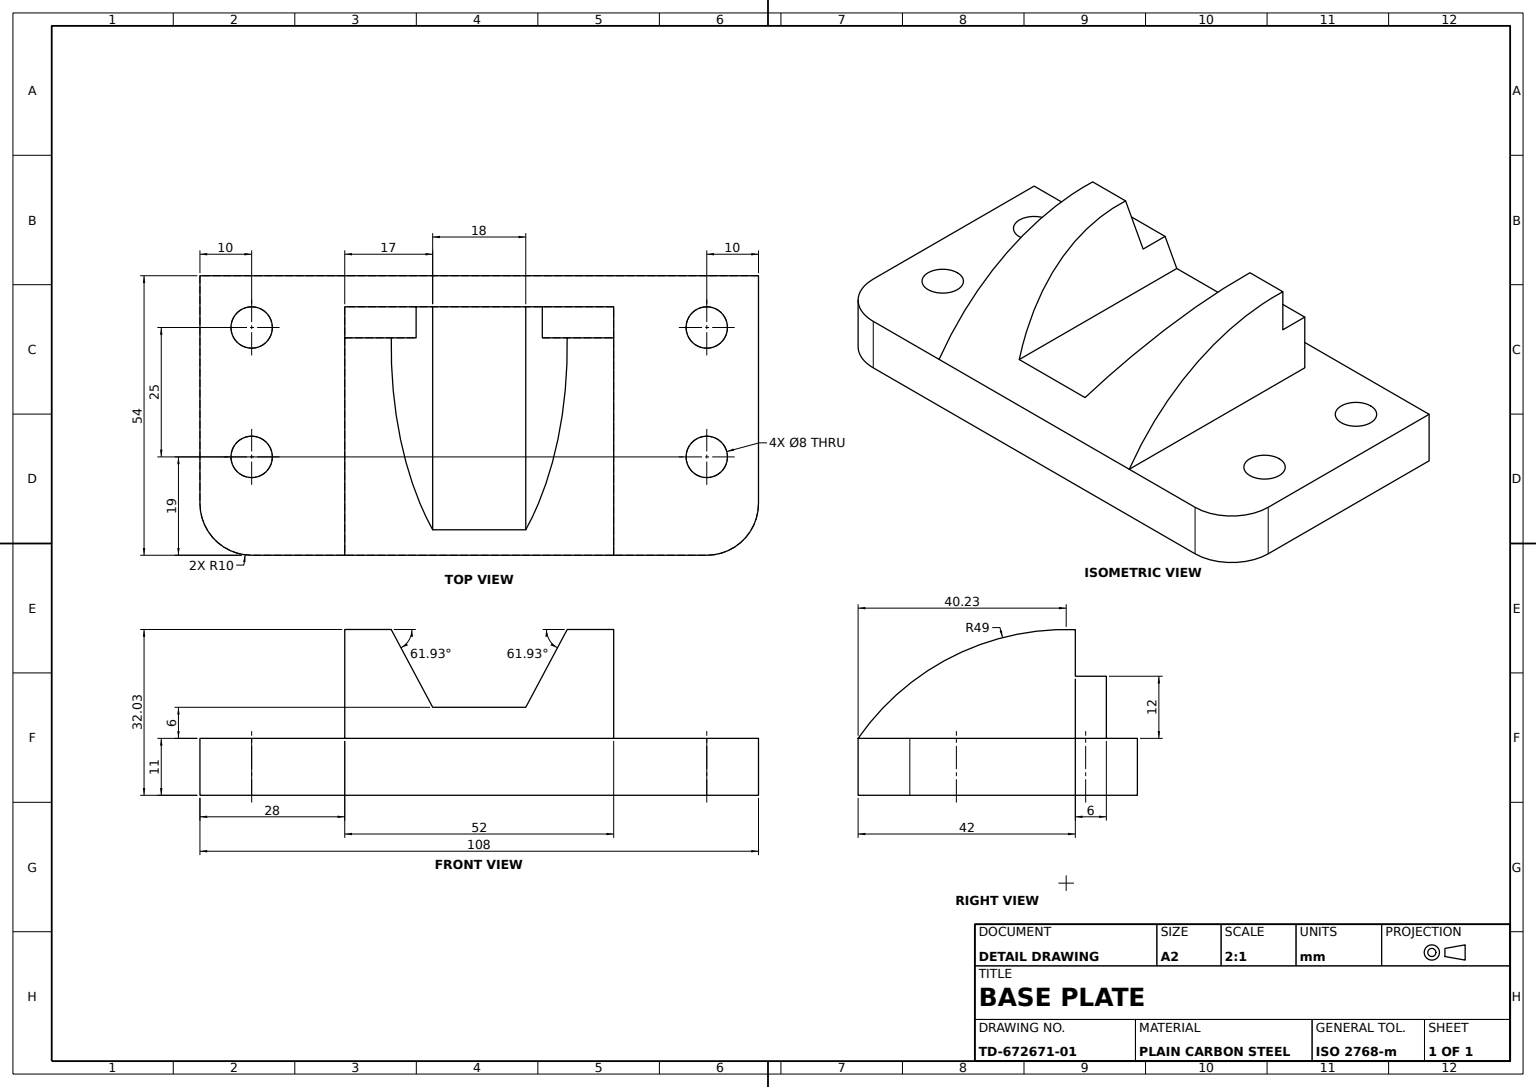
SolidWorks part; units mm, degrees
material "Plain Carbon Steel"
ref_plane "Front Plane" through (0, 0, 0) normal (0, 0, 1) x (1, 0, 0)
ref_plane "Top Plane" through (0, 0, 0) normal (0, 1, 0) x (1, 0, 0)
ref_plane "Right Plane" through (0, 0, 0) normal (1, 0, 0) x (0, 0, -1)
sketch "Base Plate Sketch" plane through (0, 0, 0) normal (0, 1, 0) x (1, 0, 0)
  line L1 (-44, -27) -> (44, -27)
  line L2 (-54, -17) -> (-54, 27)
  line L3 (-54, 27) -> (54, 27)
  line L4 (54, -17) -> (54, 27)
  circle A0 centre (-44, 17) radius 4
  circle A1 centre (-44, -8) radius 4
  circle A2 centre (44, 17) radius 4
  circle A3 centre (44, -8) radius 4
  arc A4 (44, -27) -> (54, -17) centre (44, -17) ccw
  arc A5 (-44, -27) -> (-54, -17) centre (-44, -17) cw
  point P0 (0, 0)
  point P18 (-54, -27)
  dimension "D3" = 8
  dimension "D4" = 8
  dimension "D5" = 8
  dimension "D6" = 8
  dimension "D14" = 10
  dimension "D1" = 54
  dimension "D2" = 108
  dimension "D7" = 10
  dimension "D8" = 10
  dimension "D9" = 10
  dimension "D10" = 10
  dimension "D11" = 10
  dimension "D12" = 25
  dimension "D13" = 25
  dimension "D15" = 54
  dimension "D16" = 27
extrude "Base Plate" add sketch "Base Plate Sketch" along normal blind 11
ref_plane "Plane1" through (0, 0, 0) normal (1, 0, 0) x (0, 0, -1)
ref_plane "Plane3" through (0, 0, 0) normal (0, 0, 1) x (1, 0, 0)
sketch "Saddle Block Sketch" plane through (0, 11, 0) normal (0, 1, 0) x (1, 0, 0)
  line L0 (-26, -27) -> (-26, 21)
  line L1 (-44, -27) -> (44, -27) construction
  line L2 (-26, 21) -> (26, 21)
  line L3 (26, 21) -> (26, -27)
  line L4 (26, -27) -> (-26, -27)
  line L5 (54, 27) -> (-54, 27) construction
  dimension "D1" = 52
  dimension "D2" = 26
  dimension "D3" = 6
extrude "Saddle Block" add sketch "Saddle Block Sketch" along normal blind 61
sketch "Saddle Arc Profile Sketch" plane through (26, 0, 0) normal (1, 0, 0) x (0, 0, -1)
  line L0 (15, 23) -> (15, 32)
  line L1 (21, 72) -> (21, 11) construction
  line L2 (21, 23) -> (15, 23)
  line L4 (-27, 11) -> (21, 11) construction
  line L11 (-27, 11) -> (-38.8857, 11)
  line L12 (-38.8857, 11) -> (-38.8857, 85.9595)
  line L13 (-38.8857, 85.9595) -> (45.4498, 85.9595)
  line L14 (45.4498, 85.9595) -> (44.2431, 28.3057)
  line L15 (44.2431, 28.3057) -> (21, 23)
  arc A0 (15, 32) -> (-27, 11) centre (13.2341, -16.9682) ccw
  dimension "D4" = 98
  dimension "D1" = 23.2431
  dimension "D2" = 24.4498
  dimension "D3" = 6
  dimension "D5" = 7.7659
  dimension "D6" = 59.8857
  dimension "D7" = 12
  dimension "D8" = 17.3057
  dimension "D9" = 74.9595
extrude "Saddle Arc Profile Cut" cut sketch "Saddle Arc Profile Sketch" against normal blind 61
sketch "Saddle Relief Sketch" plane through (0, 0, 27) normal (0, 0, 1) x (1, 0, 0)
  line L2 (0, 0) -> (0, 46.4301)
  line L3 (-17.017, 32.0318) -> (17.017, 32.0318)
  line L11 (-9, 17) -> (9, 17)
  line L12 (-26, 11) -> (26, 11) construction
  line L13 (-9, 17) -> (-17.017, 32.0318)
  line L14 (9, 17) -> (17.017, 32.0318)
  point P10 (0, 17)
  dimension "D4" = 21.0318
  dimension "D1" = 26.983
  dimension "D2" = 18
  dimension "D3" = 6
  dimension "D5" = 35.4301
extrude "Saddle Relief Cut" cut sketch "Saddle Relief Sketch" against normal blind 61 contours L13 L3 L14 L11
